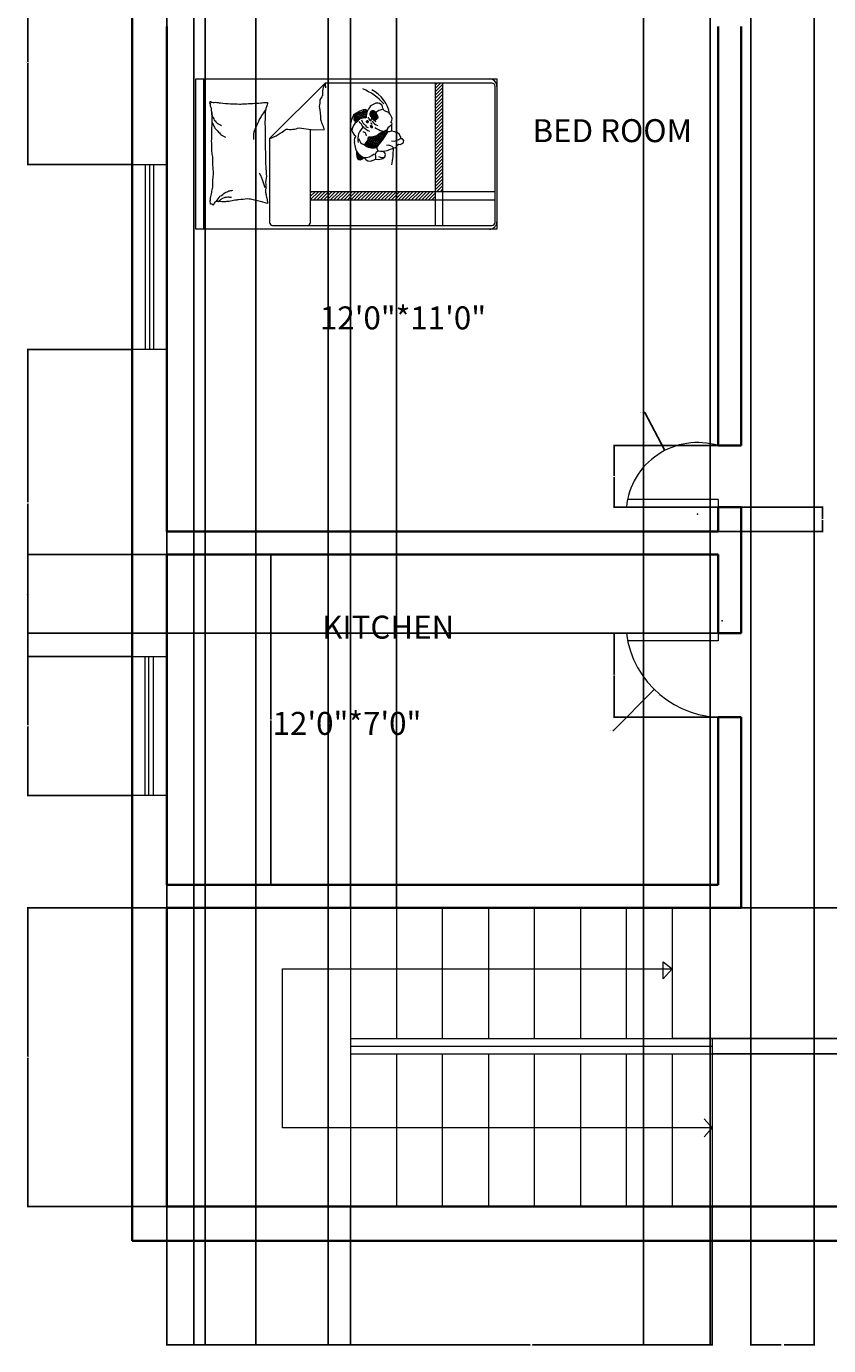
# Model space of a CAD drawing. Units: inches. Extents: x -17 to 1735, y -531 to 60.
# Tile 1 of 27: x -17 to 193, y -531 to -187. Entities that reach past the tile are written whole.
import ezdxf

# ---------------------------------------------------------------- set-up
doc = ezdxf.new("R2010")
doc.units = ezdxf.units.IN
doc.header["$MEASUREMENT"] = 0
for name, color, linetype, lineweight in [('A-ANNO-DIMS', 2, 'Continuous', 18), ('A-AREA-IDEN', 7, 'Continuous', 25), ('A-DOOR', 4, 'Continuous', 18), ('A-FLOR-STRS', 7, 'Continuous', 18), ('A-GLAZ', 4, 'Continuous', 18), ('A-WALL', 7, 'Continuous', 35)]:
    doc.layers.add(name, color=color, linetype=linetype, lineweight=lineweight)
doc.layers.add('A-FURN', color=242, linetype='Continuous', lineweight=18, true_color=0xcd2027)
doc.styles.get("Standard").update_dxf_attribs({"font": 'arial.ttf'})
doc.dimstyles.get("Standard").update_dxf_attribs({"dimtxt": 0.18, "dimasz": 0.18, "dimexe": 0.18, "dimexo": 0.0625, "dimgap": 0.09, "dimtad": 0, "dimtih": 1, "dimtoh": 1, "dimdec": 4, "dimzin": 0, "dimdsep": 46, "dimtxsty": 'Standard', "dimcen": 0.09, "dimadec": 0, "dimazin": 0, "dimtfac": 1, "dimtdec": 4, "dimtofl": 0, "dimtmove": 0, "dimatfit": 3, "dimfxl": 1, "dimtolj": 1, "dimtzin": 0, "dimarcsym": 0})

# ---------------------------------------------------------------- blocks, each defined once
blk = doc.blocks.new('BED-SINGLE-PLAN')
h = blk.add_hatch()
h.set_pattern_fill('ANSI31', color=256, scale=0.196463, angle=90, style=0)
h.set_pattern_definition([(225, (-27.0618, 48.5235), (-0.4410725, 0.4410725), [])])
h.paths.add_polyline_path([(62.55, 9.8), (29.91, 9.8), (29.91, 7.6), (62.55, 7.6)])
h.paths.add_polyline_path([(62.55, 9.8), (64.48, 9.8), (64.48, 38.18), (62.55, 38.18)])
h = blk.add_hatch()
h.set_pattern_fill('ANSI31', color=256, scale=2.357559, angle=112.8083, style=0)
h.set_pattern_definition([(157.808265, (-756.06988, 363.93155), (-0.11130837, -0.27286535), [])])
h.paths.add_polyline_path([(42.9, 28.85), (43.53, 29.05), (44.41, 29.13), (44.47, 29.42), (44.54, 30.16), (44.69, 30.7), (44.07, 30.85), (43.35, 30.52), (41.94, 30.01), (41.58, 29.54), (41.52, 28.62), (41.97, 28.11), (42.32, 28.49)])
h.paths.add_polyline_path([(45.09, 24.15, -0.19505), (43.9, 22.11, 0.242355), (47, 21.35, 0.070869), (50.1, 25.47), (49.89, 25.73), (49.62, 25.88), (48.82, 25.54), (47.87, 25.05), (47.21, 24.51), (46.36, 24.21)])
h = blk.add_hatch()
h.set_pattern_fill('ANSI31', color=256, scale=0.556973, angle=112.8083, style=0)
h.set_pattern_definition([(157.808265, (-714.60694, 367.20017), (-0.0262966024, -0.0644644387), [])])
h.paths.add_polyline_path([(45.8, 27.02), (45.59, 27), (45.47, 26.92), (45.58, 26.73), (45.73, 26.62), (46.03, 26.56), (46.14, 26.64), (46.08, 26.8), (45.97, 26.95)])
h.paths.add_polyline_path([(44.84, 28.32), (44.68, 28.33), (44.51, 28.27), (44.45, 28.18), (44.46, 28.11), (44.56, 28.01), (44.67, 27.9), (44.88, 27.87), (45.01, 27.95), (45.02, 28.12)])
h = blk.add_hatch()
h.set_pattern_fill('ANSI31', color=256, scale=1.392433, angle=112.8083, style=0)
h.set_pattern_definition([(157.808265, (-714.60694, 367.20017), (-0.065741506, -0.161161097), [])])
h.paths.add_polyline_path([(45.75, 29.39), (46.01, 28.9), (46.14, 28.75), (46.34, 28.64), (46.5, 28.59), (46.86, 28.63), (47.26, 28.84), (47.59, 29.2), (47.52, 29.53), (47.21, 29.96), (47.12, 30.29), (46.97, 30.53), (46.54, 30.87), (46.19, 31), (45.76, 30.88), (45.45, 30.56), (45.37, 30.21), (45.4, 29.92), (45.54, 29.52)])
h = blk.add_hatch()
h.set_pattern_fill('ANSI31', color=256, scale=1.178779, angle=112.8083, style=0)
h.set_pattern_definition([(157.808265, (-756.06988, 363.93155), (-0.055654185, -0.136432674), [])])
h.paths.add_polyline_path([(41.9, 20.41), (41.91, 20.39), (41.88, 19.75), (42, 19.04), (42.19, 18.52), (42.51, 18.19), (42.99, 18.18), (43.33, 18.35), (43.64, 18.6), (43.79, 18.72, -0.129501)])
for p, q in [((0, 39.29), (78.59, 39.29)), ((0, 0), (0, 39.29)), ((2.06, 0), (2.06, 39.29)), ((19.2, 23.68), (33.73, 38.18)), ((77.32, 38.18), (33.73, 38.18)), ((62.55, 1.01), (62.55, 38.18)), ((64.48, 1.01), (64.48, 38.18)), ((78.59, 39.29), (78.59, 0)), ((78.11, 1.8), (78.11, 37.39)), ((29.91, 1.8), (29.91, 26.11)), ((19.2, 23.68), (19.2, 1.8)), ((78.59, 0), (0, 0)), ((19.98, 1.01), (77.32, 1.01))]:
    blk.add_line(p, q)
for points in [[(5.25, 7.27, 0.263368), (4.51, 6.17, 0.494818), (3.78, 6.53, 0.049225), (3.71, 7.23, 0.036831), (3.78, 8.16, 0.031893), (4.1, 9.65, -0.035782), (4.37, 10.98, -0.032941), (4.6, 14.51, -0.026564), (4.37, 18.88, -0.017905), (4.16, 20.35, 0.009667), (4.07, 23.11, 0.03204), (4.1, 24.57, -0.018442), (4.22, 27.09, -0.010837), (4.19, 29.64, -0.014624), (4.07, 31.52, -0.111249), (3.78, 32.41, 0.153708), (3.63, 33.07, 0.076444), (3.7, 33.36, 0.215512), (3.78, 33.44, 0.585858), (3.9, 33.33, -0.363489), (4, 33.14, -0.191716), (4.45, 33.14, 0.129675), (5.1, 33.22, 0.01735), (5.76, 33.1, -0.019326), (6.36, 33, -0.018818), (9.04, 32.74, -0.021828), (11.37, 32.7, -0.006204), (12.7, 32.76, -0.001963), (16.9, 33, -0.028341), (18.32, 33.16, 0.117014), (18.67, 33.14, 0.36606), (18.71, 33.09, 0.03973), (18.6, 32.55, 0.048309), (18.38, 32.01, -0.062981), (18.23, 31.59, -0.04058), (18.09, 30.67, -0.014345), (18.01, 28.05, -0.005484), (18.04, 23.12, -0.004707), (18.15, 17.38, -0.008762), (18.26, 15.71, 0.008153), (18.38, 13.91, 0.06251), (18.2, 11.67, -0.078669), (18.12, 9.88, -0.047825), (18.31, 9, 0.034494), (18.6, 7.79, 0.023571), (18.71, 6.79, 0.510228), (18.67, 6.76), (17.49, 7.05), (14.25, 7.86, -0.073041), (13.48, 7.94, -0.023305), (11.08, 7.72, -0.018299), (10.18, 7.56, 0.01097), (8.68, 7.27, 0.042281), (7.34, 7.15, 0.027201), (5.24, 7.27)], [(4, 31.08, -0.088153), (4.14, 29.72, -0.088153), (4.73, 28.5, -0.077547), (5.58, 27.64, -0.077547), (6.65, 27.09)], [(18.15, 31.23, -0.016108), (17.12, 29.7, -0.024599), (16.53, 28.64, -0.009477), (15.62, 26.72, -0.015937), (15.13, 25.54, -0.072521), (14.99, 24.9, -0.033339), (14.98, 23.48)], [(4.22, 27.86, -0.027842), (4.64, 26.92, -0.048685), (4.96, 26.43, -0.023666), (5.91, 25.33, -0.031223), (6.72, 24.58, -0.046801), (7.03, 24.38, -0.023191), (7.68, 24.07)], [(19.2, 23.68, 0.085272), (23.52, 26.17, 0.124044), (26.96, 26.53), (30.71, 25.99), (33.56, 26.06)], [(18.09, 10.82, -0.009729), (17.74, 11.9, -0.009729), (17.34, 12.95, -0.007971), (16.99, 13.81, -0.007971), (16.61, 14.65)], [(5.25, 7.27, 0.077379), (6.25, 8.63, 0.077379), (7.61, 9.63, 0.047525), (8.58, 10.02, 0.047525), (9.6, 10.22)], [(5.88, 7.21, 0.05369), (6.39, 7.77, 0.070312), (6.87, 8.08, 0.015448), (7.21, 8.23, 0.013244), (7.61, 8.38, 0.082127), (8.32, 8.5, 0.064164), (9.23, 8.38)]]:
    blk.add_lwpolyline(points, format="xyb")
for points in [[(43.79, 18.72), (44.04, 18.56), (44.46, 18.12), (44.86, 17.87), (45.53, 17.83), (46.24, 18.04), (46.92, 18.32), (47.57, 18.24), (48.51, 18.4), (48.81, 18.47), (49.3, 18.91), (49.47, 19.49), (49.29, 19.97), (48.92, 20.38), (49.91, 20.56), (51.05, 21.01), (51.55, 21.16), (51.59, 21.33), (51.88, 21.27), (52.46, 21.66), (52.55, 22), (52.94, 22.19), (53.35, 22.15), (53.8, 22.4), (54.07, 22.6), (54.21, 22.84), (54.27, 23.19), (53.95, 23.59), (53.59, 23.67), (53.53, 23.82), (53.51, 24.14), (53.22, 24.49), (53.14, 24.75), (52.57, 25.26), (52.25, 25.24), (51.94, 25.49), (50.98, 25.59), (50.47, 25.47), (50.13, 25.44), (49.89, 25.73), (49.62, 25.88), (49.97, 26.17), (50.19, 26.42), (50.21, 26.66), (50.65, 26.93), (50.88, 27.18), (51.12, 27.37), (51.24, 27.65), (51.14, 27.82), (50.96, 27.83), (50.98, 28.05), (51.12, 28.43), (51.19, 28.96), (51.17, 29.16), (50.93, 29.59), (50.71, 30.03), (50.42, 30.38), (49.9, 30.7), (49.25, 30.9), (49.09, 31.16), (48.83, 31.61), (48.74, 31.98), (48.58, 32.42), (47.95, 32.87), (47.57, 32.94), (46.99, 32.91), (46.24, 32.59), (45.6, 32.26), (45.31, 31.84), (44.99, 31.21), (44.78, 31), (44.17, 31.25), (43.66, 31.18), (42.75, 30.83), (42.33, 30.56), (41.65, 30.22), (41.1, 29.84), (40.84, 29.19), (40.62, 28.57), (40.38, 27.67), (40.38, 26.55), (40.44, 26.19), (40.7, 25.86), (40.89, 25.34), (41.33, 24.64), (41.74, 24.31), (41.36, 23.8), (41.32, 23.27), (41.4, 23.13), (41.29, 22.64), (41.54, 21.48), (41.64, 21.02), (41.71, 20.72), (41.85, 20.54), (41.91, 20.39), (41.88, 19.75), (42, 19.04), (42.19, 18.52), (42.51, 18.19), (42.99, 18.18), (43.33, 18.35), (43.64, 18.6), (43.79, 18.72)], [(41.81, 27.96), (41.3, 28.55), (41.37, 29.62), (41.81, 30.2), (43.27, 30.72), (44.05, 31.08), (44.74, 30.91)], [(41.97, 28.11), (41.52, 28.62), (41.58, 29.54), (41.94, 30.01), (43.35, 30.52), (44.07, 30.85), (44.69, 30.7)], [(44.78, 31), (44.54, 30.16), (44.47, 29.42), (44.41, 29.13), (43.53, 29.05), (42.9, 28.85), (42.32, 28.49), (41.97, 28.11)], [(44.67, 27.9), (44.88, 27.87), (45.01, 27.95), (45.02, 28.12), (44.84, 28.32), (44.68, 28.33), (44.51, 28.27), (44.45, 28.18), (44.46, 28.11), (44.56, 28.01), (44.67, 27.9)], [(45.75, 29.39), (46.01, 28.9), (46.14, 28.75), (46.34, 28.64), (46.5, 28.59), (46.86, 28.63), (47.26, 28.84), (47.59, 29.2), (47.52, 29.53), (47.21, 29.96), (47.12, 30.29), (46.97, 30.53), (46.54, 30.87), (46.19, 31), (45.76, 30.88), (45.45, 30.56), (45.37, 30.21), (45.4, 29.92), (45.54, 29.52), (45.75, 29.39)], [(45.09, 24.15), (46.36, 24.21), (47.21, 24.51), (47.87, 25.05), (48.82, 25.54), (49.62, 25.88)], [(45.73, 26.62), (46.03, 26.56), (46.14, 26.64), (46.08, 26.8), (45.97, 26.95), (45.8, 27.02), (45.59, 27), (45.47, 26.92), (45.58, 26.73), (45.73, 26.62)], [(46.92, 18.32), (46.96, 18.99), (46.83, 19.65), (47.14, 20.19), (47.67, 20.47), (48.14, 20.41), (48.92, 20.38)], [(78.11, 9.8), (29.91, 9.8)], [(78.11, 7.6), (29.91, 7.6)]]:
    blk.add_lwpolyline(points)
for centre, radius, start, end in [((38, 35.55), 5.01, 148.4201, 187.4443), ((39.59, 38.03), 5.86, 178.5957, 190.5745), ((76.62, 37.33), 1.96, 0, 90), ((77.32, 37.39), 0.786, 0, 90), ((30.16, 35.71), 2.97, 320.6139, 344.2839), ((38.03, 23.16), 14.6, 41.0314, 67.8934), ((42.02, 28.67), 8.66, 9.4371, 63.5432), ((26.72, 33.64), 5.74, 344.2839, 1.7887), ((10.08, 27.94), 22.56, 1.7887, 10.5945), ((49.55, 27.35), 4.08, 98.3054, 168.9473), ((26.25, 26.33), 6.78, 10.5945, 19.9478), ((19.4, 20.92), 15.06, 19.9478, 26.2172), ((44.35, 25.28), 3.69, 130.0646, 171.0184), ((40.73, 25.75), 3, 17.6284, 51.9822), ((45.01, 28.9), 1.81, 191.014, 241.9838), ((46.38, 29.75), 1.54, 196.6236, 237.032), ((46.1, 27.86), 0.431, 180.1097, 257.3601), ((46.45, 29.64), 0.695, 97.7782, 185.1837), ((45.99, 30.23), 0.379, 14.3938, 104.927), ((48.22, 29.75), 2.7, 214.8006, 254.2713), ((46.73, 29.37), 0.572, 4.9536, 167.0589), ((54.94, 39.79), 14.12, 231.9927, 235.4886), ((46.6, 29.87), 0.512, 10.7395, 118.1073), ((46.27, 23.6), 4.03, 126.6141, 193.9334), ((43.31, 24.26), 1.25, 5.5542, 75.9589), ((47.07, 29.65), 4.44, 223.4778, 246.0857), ((41.98, 24.59), 3.13, 307.7547, 351.9024), ((44.99, 27.32), 0.729, 184.2478, 266.558), ((49.36, 29.79), 4.14, 230.1138, 260.2426), ((34.07, 34.29), 18.29, 314.9707, 331.1855), ((11.77, 25.26), 39.39, 0.4734, 3.0628), ((46.04, 23.16), 4.97, 209.3586, 243.0552), ((44.61, 24.23), 2.23, 194.7325, 251.4551), ((46.2, 24.74), 3.49, 228.8697, 283.3627), ((48.1, 21.24), 0.883, 163.0797, 240.2757), ((50.18, 20.2), 1.73, 36.8303, 104.4951), ((51.66, 25.7), 2.65, 256.5554, 314.9062), ((29.44, 21.14), 22.11, 348.8153, 0.0463), ((44.02, 22.54), 3.83, 266.6283, 311.5254), ((48.58, 20.29), 1.56, 234.8325, 297.5513), ((19.98, 1.8), 0.786, 180, 270), ((29.12, 1.8), 0.786, 270, 0), ((76.62, 1.96), 1.96, 270, 0), ((77.32, 1.8), 0.786, 270, 0)]:
    blk.add_arc(centre, radius, start, end)
blk = doc.blocks.new('WIN-FRAME-48IN')
for p, q in [((3.31, 48.33), (3.31, 0)), ((5.59, 0), (5.59, 48.33))]:
    blk.add_line(p, q)
blk.add_lwpolyline([(0, 48.33), (9, 48.33), (9, 0), (0, 0)], close=True)
blk = doc.blocks.new('*D11')
at = {"layer": 'A-ANNO-DIMS', "color": 0, "lineweight": -2, "transparency": 16777216}
for p, q in [((20.06, 23.17), (20.06, -531.46)), ((62.23, 23.17), (62.23, -531.46)), ((20.24, -531.28), (40.75, -531.28)), ((62.05, -531.28), (41.54, -531.28))]:
    blk.add_line(p, q, dxfattribs=at)
at = {"layer": 'A-ANNO-DIMS', "color": 0, "transparency": 16777216}
for points in [[(20.24, -531.25), (20.24, -531.31), (20.06, -531.28)], [(62.05, -531.25), (62.05, -531.31), (62.23, -531.28)]]:
    blk.add_solid(points, dxfattribs=at)
at = {"layer": 'Defpoints', "color": 0, "transparency": 16777216}
for p in [(20.06, 23.23), (62.23, 23.23), (62.23, -531.28)]:
    blk.add_point(p, dxfattribs=at)
at = {"layer": 'A-ANNO-DIMS', "color": 0, "transparency": 16777216, "insert": (41.15, -531.28), "char_height": 0.18, "attachment_point": 5}
blk.add_mtext('\\A1;42.17', dxfattribs=at)
blk = doc.blocks.new('*D15')
at = {"layer": 'A-ANNO-DIMS', "color": 0, "lineweight": -2, "transparency": 16777216}
for p, q in [((11, -169.55), (-16.4, -169.55)), ((-16.22, -169.73), (-16.22, -196.03)), ((-16.22, -222.7), (-16.22, -196.39)), ((11, -222.88), (-16.4, -222.88))]:
    blk.add_line(p, q, dxfattribs=at)
at = {"layer": 'A-ANNO-DIMS', "color": 0, "transparency": 16777216}
for points in [[(-16.25, -169.73), (-16.19, -169.73), (-16.22, -169.55)], [(-16.25, -222.7), (-16.19, -222.7), (-16.22, -222.88)]]:
    blk.add_solid(points, dxfattribs=at)
at = {"layer": 'Defpoints', "color": 0, "transparency": 16777216}
for p in [(11.06, -169.55), (-16.22, -222.88), (11.06, -222.88)]:
    blk.add_point(p, dxfattribs=at)
at = {"layer": 'A-ANNO-DIMS', "color": 0, "transparency": 16777216, "insert": (-16.22, -196.21), "char_height": 0.18, "attachment_point": 5}
blk.add_mtext('\\A1;53.33', dxfattribs=at)
blk = doc.blocks.new('*D16')
at = {"layer": 'A-ANNO-DIMS', "color": 0, "lineweight": -2, "transparency": 16777216}
for p, q in [((11, -271.2), (-16.4, -271.2)), ((-16.22, -271.38), (-16.22, -311.12)), ((-16.22, -351.23), (-16.22, -311.49)), ((10.91, -351.41), (-16.4, -351.41))]:
    blk.add_line(p, q, dxfattribs=at)
at = {"layer": 'A-ANNO-DIMS', "color": 0, "transparency": 16777216}
for points in [[(-16.25, -271.38), (-16.19, -271.38), (-16.22, -271.2)], [(-16.25, -351.23), (-16.19, -351.23), (-16.22, -351.41)]]:
    blk.add_solid(points, dxfattribs=at)
at = {"layer": 'Defpoints', "color": 0, "transparency": 16777216}
for p in [(11.06, -271.2), (-16.22, -351.41), (10.98, -351.41)]:
    blk.add_point(p, dxfattribs=at)
at = {"layer": 'A-ANNO-DIMS', "color": 0, "transparency": 16777216, "insert": (-16.22, -311.3), "char_height": 0.18, "attachment_point": 5}
blk.add_mtext('\\A1;80.2', dxfattribs=at)
blk = doc.blocks.new('*D17')
at = {"layer": 'A-ANNO-DIMS', "color": 0, "lineweight": -2, "transparency": 16777216}
for p, q in [((10.91, -351.41), (-16.4, -351.41)), ((-16.22, -351.59), (-16.22, -369.37)), ((-16.22, -387.51), (-16.22, -369.73)), ((10.91, -387.69), (-16.4, -387.69))]:
    blk.add_line(p, q, dxfattribs=at)
at = {"layer": 'A-ANNO-DIMS', "color": 0, "transparency": 16777216}
for points in [[(-16.25, -351.59), (-16.19, -351.59), (-16.22, -351.41)], [(-16.25, -387.51), (-16.19, -387.51), (-16.22, -387.69)]]:
    blk.add_solid(points, dxfattribs=at)
at = {"layer": 'Defpoints', "color": 0, "transparency": 16777216}
for p in [(10.98, -351.41), (-16.22, -387.69), (10.98, -387.69)]:
    blk.add_point(p, dxfattribs=at)
at = {"layer": 'A-ANNO-DIMS', "color": 0, "transparency": 16777216, "insert": (-16.22, -369.55), "char_height": 0.18, "attachment_point": 5}
blk.add_mtext('\\A1;36.28', dxfattribs=at)
blk = doc.blocks.new('*D30')
at = {"layer": 'A-ANNO-DIMS', "color": 0, "lineweight": -2, "transparency": 16777216}
for p, q in [((144.53, -126.83), (144.53, -531.46)), ((161.94, -126.83), (161.94, -531.46)), ((144.71, -531.28), (152.87, -531.28)), ((161.76, -531.28), (153.6, -531.28))]:
    blk.add_line(p, q, dxfattribs=at)
at = {"layer": 'A-ANNO-DIMS', "color": 0, "transparency": 16777216}
for points in [[(144.71, -531.25), (144.71, -531.31), (144.53, -531.28)], [(161.76, -531.25), (161.76, -531.31), (161.94, -531.28)]]:
    blk.add_solid(points, dxfattribs=at)
at = {"layer": 'Defpoints', "color": 0, "transparency": 16777216}
for p in [(144.53, -126.77), (161.94, -126.77), (161.94, -531.28)]:
    blk.add_point(p, dxfattribs=at)
at = {"layer": 'A-ANNO-DIMS', "color": 0, "transparency": 16777216, "insert": (153.23, -531.28), "char_height": 0.18, "attachment_point": 5}
blk.add_mtext('\\A1;17.41', dxfattribs=at)
blk = doc.blocks.new('*D31')
at = {"layer": 'A-ANNO-DIMS', "color": 0, "lineweight": -2, "transparency": 16777216}
for p, q in [((172.55, -126.83), (172.55, -531.46)), ((189.13, -126.83), (189.13, -531.46)), ((172.73, -531.28), (180.46, -531.28)), ((188.95, -531.28), (181.23, -531.28))]:
    blk.add_line(p, q, dxfattribs=at)
at = {"layer": 'A-ANNO-DIMS', "color": 0, "transparency": 16777216}
for points in [[(172.73, -531.25), (172.73, -531.31), (172.55, -531.28)], [(188.95, -531.25), (188.95, -531.31), (189.13, -531.28)]]:
    blk.add_solid(points, dxfattribs=at)
at = {"layer": 'Defpoints', "color": 0, "transparency": 16777216}
for p in [(172.55, -126.77), (189.13, -126.77), (189.13, -531.28)]:
    blk.add_point(p, dxfattribs=at)
at = {"layer": 'A-ANNO-DIMS', "color": 0, "transparency": 16777216, "insert": (180.84, -531.28), "char_height": 0.18, "attachment_point": 5}
blk.add_mtext('\\A1;16.58', dxfattribs=at)
blk = doc.blocks.new('*D33')
at = {"layer": 'A-ANNO-DIMS', "color": 0, "lineweight": -2, "transparency": 16777216}
for p, q in [((164, -296.3), (136.68, -296.3)), ((136.86, -296.48), (136.86, -304.18)), ((136.86, -312.24), (136.86, -304.54)), ((164, -312.42), (136.68, -312.42))]:
    blk.add_line(p, q, dxfattribs=at)
at = {"layer": 'A-ANNO-DIMS', "color": 0, "transparency": 16777216}
for points in [[(136.83, -296.48), (136.89, -296.48), (136.86, -296.3)], [(136.83, -312.24), (136.89, -312.24), (136.86, -312.42)]]:
    blk.add_solid(points, dxfattribs=at)
at = {"layer": 'Defpoints', "color": 0, "transparency": 16777216}
for p in [(136.86, -296.3), (164.06, -296.3), (164.06, -312.42)]:
    blk.add_point(p, dxfattribs=at)
at = {"layer": 'A-ANNO-DIMS', "color": 0, "transparency": 16777216, "insert": (136.86, -304.36), "char_height": 0.18, "attachment_point": 5}
blk.add_mtext('\\A1;16.116', dxfattribs=at)
blk = doc.blocks.new('*D34')
at = {"layer": 'A-ANNO-DIMS', "color": 0, "lineweight": -2, "transparency": 16777216}
for p, q in [((164.12, -312.42), (191.44, -312.42)), ((191.26, -312.6), (191.26, -315.41)), ((191.26, -318.59), (191.26, -315.78)), ((164.12, -318.77), (191.44, -318.77))]:
    blk.add_line(p, q, dxfattribs=at)
at = {"layer": 'A-ANNO-DIMS', "color": 0, "transparency": 16777216}
for points in [[(191.23, -312.6), (191.29, -312.6), (191.26, -312.42)], [(191.23, -318.59), (191.29, -318.59), (191.26, -318.77)]]:
    blk.add_solid(points, dxfattribs=at)
at = {"layer": 'Defpoints', "color": 0, "transparency": 16777216}
for p in [(164.06, -312.42), (164.06, -318.77), (191.26, -318.77)]:
    blk.add_point(p, dxfattribs=at)
at = {"layer": 'A-ANNO-DIMS', "color": 0, "transparency": 16777216, "insert": (191.26, -315.59), "char_height": 0.18, "attachment_point": 5}
blk.add_mtext('\\A1;6.351', dxfattribs=at)
blk = doc.blocks.new('*D35')
at = {"layer": 'A-ANNO-DIMS', "color": 0, "lineweight": -2, "transparency": 16777216}
for p, q in [((164, -324.77), (-16.4, -324.77)), ((-16.22, -324.95), (-16.22, -334.86)), ((-16.22, -345.14), (-16.22, -335.23)), ((164, -345.32), (-16.4, -345.32))]:
    blk.add_line(p, q, dxfattribs=at)
at = {"layer": 'A-ANNO-DIMS', "color": 0, "transparency": 16777216}
for points in [[(-16.25, -324.95), (-16.19, -324.95), (-16.22, -324.77)], [(-16.25, -345.14), (-16.19, -345.14), (-16.22, -345.32)]]:
    blk.add_solid(points, dxfattribs=at)
at = {"layer": 'Defpoints', "color": 0, "transparency": 16777216}
for p in [(-16.22, -324.77), (164.06, -324.77), (164.06, -345.32)]:
    blk.add_point(p, dxfattribs=at)
at = {"layer": 'A-ANNO-DIMS', "color": 0, "transparency": 16777216, "insert": (-16.22, -335.04), "char_height": 0.18, "attachment_point": 5}
blk.add_mtext('\\A1;20.553', dxfattribs=at)
blk = doc.blocks.new('*D36')
at = {"layer": 'A-ANNO-DIMS', "color": 0, "lineweight": -2, "transparency": 16777216}
for p, q in [((164, -345.32), (136.68, -345.32)), ((136.86, -345.5), (136.86, -356.1)), ((136.86, -367.06), (136.86, -356.46)), ((164, -367.24), (136.68, -367.24))]:
    blk.add_line(p, q, dxfattribs=at)
at = {"layer": 'A-ANNO-DIMS', "color": 0, "transparency": 16777216}
for points in [[(136.83, -345.5), (136.89, -345.5), (136.86, -345.32)], [(136.83, -367.06), (136.89, -367.06), (136.86, -367.24)]]:
    blk.add_solid(points, dxfattribs=at)
at = {"layer": 'Defpoints', "color": 0, "transparency": 16777216}
for p in [(136.86, -345.32), (164.06, -345.32), (164.06, -367.24)]:
    blk.add_point(p, dxfattribs=at)
at = {"layer": 'A-ANNO-DIMS', "color": 0, "transparency": 16777216, "insert": (136.86, -356.28), "char_height": 0.18, "attachment_point": 5}
blk.add_mtext('\\A1;21.923', dxfattribs=at)
blk = doc.blocks.new('*D42')
at = {"layer": 'A-ANNO-DIMS', "color": 0, "lineweight": -2, "transparency": 16777216}
for p, q in [((20.12, -324.77), (47.44, -324.77)), ((47.26, -324.95), (47.26, -367.74)), ((47.26, -410.9), (47.26, -368.11)), ((20.12, -411.08), (47.44, -411.08))]:
    blk.add_line(p, q, dxfattribs=at)
at = {"layer": 'A-ANNO-DIMS', "color": 0, "transparency": 16777216}
for points in [[(47.23, -324.95), (47.29, -324.95), (47.26, -324.77)], [(47.23, -410.9), (47.29, -410.9), (47.26, -411.08)]]:
    blk.add_solid(points, dxfattribs=at)
at = {"layer": 'Defpoints', "color": 0, "transparency": 16777216}
for p in [(20.06, -324.77), (20.06, -411.08), (47.26, -411.08)]:
    blk.add_point(p, dxfattribs=at)
at = {"layer": 'A-ANNO-DIMS', "color": 0, "transparency": 16777216, "insert": (47.26, -367.92), "char_height": 0.18, "attachment_point": 5}
blk.add_mtext('\\A1;86.31', dxfattribs=at)
blk = doc.blocks.new('*D45')
at = {"layer": 'A-ANNO-DIMS', "color": 0, "lineweight": -2, "transparency": 16777216}
for p, q in [((27.16, -164.32), (27.16, -531.46)), ((43.3, -164.32), (43.3, -531.46)), ((27.34, -531.28), (34.85, -531.28)), ((43.12, -531.28), (35.62, -531.28))]:
    blk.add_line(p, q, dxfattribs=at)
at = {"layer": 'A-ANNO-DIMS', "color": 0, "transparency": 16777216}
for points in [[(27.34, -531.25), (27.34, -531.31), (27.16, -531.28)], [(43.12, -531.25), (43.12, -531.31), (43.3, -531.28)]]:
    blk.add_solid(points, dxfattribs=at)
at = {"layer": 'Defpoints', "color": 0, "transparency": 16777216}
for p in [(27.16, -164.25), (43.3, -164.25), (43.3, -531.28)]:
    blk.add_point(p, dxfattribs=at)
at = {"layer": 'A-ANNO-DIMS', "color": 0, "transparency": 16777216, "insert": (35.23, -531.28), "char_height": 0.18, "attachment_point": 5}
blk.add_mtext('\\A1;16.14', dxfattribs=at)
blk = doc.blocks.new('*D46')
at = {"layer": 'A-ANNO-DIMS', "color": 0, "lineweight": -2, "transparency": 16777216}
for p, q in [((30.1, -177.39), (30.1, -531.46)), ((20.06, -180.83), (20.06, -531.46)), ((20.24, -531.28), (24.62, -531.28)), ((29.92, -531.28), (25.53, -531.28))]:
    blk.add_line(p, q, dxfattribs=at)
at = {"layer": 'A-ANNO-DIMS', "color": 0, "transparency": 16777216}
for points in [[(20.24, -531.25), (20.24, -531.31), (20.06, -531.28)], [(29.92, -531.25), (29.92, -531.31), (30.1, -531.28)]]:
    blk.add_solid(points, dxfattribs=at)
at = {"layer": 'Defpoints', "color": 0, "transparency": 16777216}
for p in [(30.1, -177.33), (20.06, -180.77), (30.1, -531.28)]:
    blk.add_point(p, dxfattribs=at)
at = {"layer": 'A-ANNO-DIMS', "color": 0, "transparency": 16777216, "insert": (25.08, -531.28), "char_height": 0.18, "attachment_point": 5}
blk.add_mtext('\\A1;10.034', dxfattribs=at)
blk = doc.blocks.new('*D47')
at = {"layer": 'A-ANNO-DIMS', "color": 0, "lineweight": -2, "transparency": 16777216}
for p, q in [((20, -417.08), (-16.4, -417.08)), ((-16.22, -417.26), (-16.22, -455.9)), ((-16.22, -494.9), (-16.22, -456.26)), ((20, -495.08), (-16.4, -495.08))]:
    blk.add_line(p, q, dxfattribs=at)
at = {"layer": 'A-ANNO-DIMS', "color": 0, "transparency": 16777216}
for points in [[(-16.25, -417.26), (-16.19, -417.26), (-16.22, -417.08)], [(-16.25, -494.9), (-16.19, -494.9), (-16.22, -495.08)]]:
    blk.add_solid(points, dxfattribs=at)
at = {"layer": 'Defpoints', "color": 0, "transparency": 16777216}
for p in [(-16.22, -417.08), (20.06, -417.08), (20.06, -495.08)]:
    blk.add_point(p, dxfattribs=at)
at = {"layer": 'A-ANNO-DIMS', "color": 0, "transparency": 16777216, "insert": (-16.22, -456.08), "char_height": 0.18, "attachment_point": 5}
blk.add_mtext('\\A1;78', dxfattribs=at)
blk = doc.blocks.new('*D48')
at = {"layer": 'A-ANNO-DIMS', "color": 0, "lineweight": -2, "transparency": 16777216}
for p, q in [((20.06, -495.14), (20.06, -531.46)), ((68.06, -495.14), (68.06, -531.46)), ((20.24, -531.28), (43.84, -531.28)), ((67.88, -531.28), (44.28, -531.28))]:
    blk.add_line(p, q, dxfattribs=at)
at = {"layer": 'A-ANNO-DIMS', "color": 0, "transparency": 16777216}
for points in [[(20.24, -531.25), (20.24, -531.31), (20.06, -531.28)], [(67.88, -531.25), (67.88, -531.31), (68.06, -531.28)]]:
    blk.add_solid(points, dxfattribs=at)
at = {"layer": 'Defpoints', "color": 0, "transparency": 16777216}
for p in [(20.06, -495.08), (68.06, -495.08), (68.06, -531.28)]:
    blk.add_point(p, dxfattribs=at)
at = {"layer": 'A-ANNO-DIMS', "color": 0, "transparency": 16777216, "insert": (44.06, -531.28), "char_height": 0.18, "attachment_point": 5}
blk.add_mtext('\\A1;48', dxfattribs=at)
blk = doc.blocks.new('*D49')
at = {"layer": 'A-ANNO-DIMS', "color": 0, "lineweight": -2, "transparency": 16777216}
for p, q in [((68.06, -495.14), (68.06, -531.46)), ((162.47, -495.14), (162.47, -531.46)), ((68.24, -531.28), (114.94, -531.28)), ((162.29, -531.28), (115.59, -531.28))]:
    blk.add_line(p, q, dxfattribs=at)
at = {"layer": 'A-ANNO-DIMS', "color": 0, "transparency": 16777216}
for points in [[(68.24, -531.25), (68.24, -531.31), (68.06, -531.28)], [(162.29, -531.25), (162.29, -531.31), (162.47, -531.28)]]:
    blk.add_solid(points, dxfattribs=at)
at = {"layer": 'Defpoints', "color": 0, "transparency": 16777216}
for p in [(68.06, -495.08), (162.47, -495.08), (162.47, -531.28)]:
    blk.add_point(p, dxfattribs=at)
at = {"layer": 'A-ANNO-DIMS', "color": 0, "transparency": 16777216, "insert": (115.26, -531.28), "char_height": 0.18, "attachment_point": 5}
blk.add_mtext('\\A1;94.4', dxfattribs=at)
blk = doc.blocks.new('*D50')
at = {"layer": 'A-ANNO-DIMS', "color": 0, "lineweight": -2, "transparency": 16777216}
for p, q in [((68.06, -417.02), (68.06, 59.62)), ((68.24, 59.44), (73.85, 59.44)), ((79.88, 59.44), (74.27, 59.44)), ((80.06, -417.02), (80.06, 59.62))]:
    blk.add_line(p, q, dxfattribs=at)
at = {"layer": 'A-ANNO-DIMS', "color": 0, "transparency": 16777216}
for points in [[(68.24, 59.47), (68.24, 59.41), (68.06, 59.44)], [(79.88, 59.47), (79.88, 59.41), (80.06, 59.44)]]:
    blk.add_solid(points, dxfattribs=at)
at = {"layer": 'Defpoints', "color": 0, "transparency": 16777216}
for p in [(80.06, 59.44), (68.06, -417.08), (80.06, -417.08)]:
    blk.add_point(p, dxfattribs=at)
at = {"layer": 'A-ANNO-DIMS', "color": 0, "transparency": 16777216, "insert": (74.06, 59.44), "char_height": 0.18, "attachment_point": 5}
blk.add_mtext('\\A1;12', dxfattribs=at)
blk = doc.blocks.new('*D51')
at = {"layer": 'A-ANNO-DIMS', "color": 0, "lineweight": -2, "transparency": 16777216}
for p, q in [((152.12, -417.08), (356.44, -417.08)), ((356.26, -417.26), (356.26, -433.97)), ((356.26, -451.04), (356.26, -434.33)), ((152.12, -451.22), (356.44, -451.22))]:
    blk.add_line(p, q, dxfattribs=at)
at = {"layer": 'A-ANNO-DIMS', "color": 0, "transparency": 16777216}
for points in [[(356.23, -417.26), (356.29, -417.26), (356.26, -417.08)], [(356.23, -451.04), (356.29, -451.04), (356.26, -451.22)]]:
    blk.add_solid(points, dxfattribs=at)
at = {"layer": 'Defpoints', "color": 0, "transparency": 16777216}
for p in [(152.06, -417.08), (152.06, -451.22), (356.26, -451.22)]:
    blk.add_point(p, dxfattribs=at)
at = {"layer": 'A-ANNO-DIMS', "color": 0, "transparency": 16777216, "insert": (356.26, -434.15), "char_height": 0.18, "attachment_point": 5}
blk.add_mtext('\\A1;34.14', dxfattribs=at)
blk = doc.blocks.new('*D52')
at = {"layer": 'A-ANNO-DIMS', "color": 0, "lineweight": -2, "transparency": 16777216}
for p, q in [((162.53, -455.22), (356.44, -455.22)), ((356.26, -455.4), (356.26, -474.97)), ((356.26, -494.9), (356.26, -475.33)), ((162.53, -495.08), (356.44, -495.08))]:
    blk.add_line(p, q, dxfattribs=at)
at = {"layer": 'A-ANNO-DIMS', "color": 0, "transparency": 16777216}
for points in [[(356.23, -455.4), (356.29, -455.4), (356.26, -455.22)], [(356.23, -494.9), (356.29, -494.9), (356.26, -495.08)]]:
    blk.add_solid(points, dxfattribs=at)
at = {"layer": 'Defpoints', "color": 0, "transparency": 16777216}
for p in [(162.47, -455.22), (162.47, -495.08), (356.26, -495.08)]:
    blk.add_point(p, dxfattribs=at)
at = {"layer": 'A-ANNO-DIMS', "color": 0, "transparency": 16777216, "insert": (356.26, -475.15), "char_height": 0.18, "attachment_point": 5}
blk.add_mtext('\\A1;39.86', dxfattribs=at)
blk = doc.blocks.new('*D56')
at = {"layer": 'A-ANNO-DIMS', "color": 0, "lineweight": -2, "transparency": 16777216}
for p, q in [((144.74, -287.64), (144.92, -287.64)), ((144.92, -287.64), (149.99, -297.44)), ((158.58, -314.2), (158.76, -314.2)), ((158.67, -314.29), (158.67, -314.11))]:
    blk.add_line(p, q, dxfattribs=at)
at = {"layer": 'A-ANNO-DIMS', "color": 0, "transparency": 16777216}
blk.add_solid([(150.02, -297.43), (149.96, -297.45), (150.07, -297.6)], dxfattribs=at)
at = {"layer": 'Defpoints', "color": 0, "transparency": 16777216}
for p in [(150.07, -297.6), (158.67, -314.2)]:
    blk.add_point(p, dxfattribs=at)
at = {"layer": 'A-ANNO-DIMS', "color": 0, "transparency": 16777216, "insert": (144.19, -287.64), "char_height": 0.18, "attachment_point": 5}
blk.add_mtext('\\A1;R18.693', dxfattribs=at)
blk = doc.blocks.new('*D57')
at = {"layer": 'A-ANNO-DIMS', "color": 0, "lineweight": -2, "transparency": 16777216}
for p, q in [((164.95, -342.07), (165.13, -342.07)), ((165.04, -342.16), (165.04, -341.98)), ((136.73, -370.76), (147.22, -360.13)), ((136.55, -370.76), (136.73, -370.76))]:
    blk.add_line(p, q, dxfattribs=at)
at = {"layer": 'A-ANNO-DIMS', "color": 0, "transparency": 16777216}
blk.add_solid([(147.2, -360.11), (147.24, -360.15), (147.35, -360)], dxfattribs=at)
at = {"layer": 'Defpoints', "color": 0, "transparency": 16777216}
for p in [(165.04, -342.07), (147.35, -360)]:
    blk.add_point(p, dxfattribs=at)
at = {"layer": 'A-ANNO-DIMS', "color": 0, "transparency": 16777216, "insert": (136.07, -370.76), "char_height": 0.18, "attachment_point": 5}
blk.add_mtext('\\A1;R25.19', dxfattribs=at)

msp = doc.modelspace()

# ---------------------------------------------------------------- linework, layer by layer
at = {"layer": 'A-DOOR'}
for p, q in [((164.0618, -312.4176), (140.0618, -312.4176)), ((164.0618, -310.4176), (140.3633, -310.4176)), ((164.0618, -310.4176), (164.0618, -312.4176)), ((164.0618, -345.3213), (140.0618, -345.3213)), ((164.0618, -347.3213), (140.4044, -347.3213)), ((164.0618, -345.3213), (164.0618, -347.3213))]:
    msp.add_line(p, q, dxfattribs=at)
for centre, radius, start, end in [((158.6693, -314.1999), 18.6927, 73.232883, 174.528677), ((165.0435, -342.0715), 25.1923, 187.411932, 272.233429)]:
    msp.add_arc(centre, radius, start, end, dxfattribs=at)
at = {"layer": 'A-FLOR-STRS'}
for p, q in [((68.0618, -417.0795), (68.0618, -495.0795)), ((80.0618, -417.0795), (80.0618, -451.2168)), ((92.0618, -417.0795), (104.0618, -417.0795)), ((92.0618, -451.2168), (92.0618, -417.0795)), ((104.0618, -417.0795), (104.0618, -451.2168)), ((116.0618, -417.0795), (128.0618, -417.0795)), ((116.0618, -451.2168), (116.0618, -417.0795)), ((128.0618, -417.0795), (128.0618, -451.2168)), ((140.0618, -417.0795), (152.0618, -417.0795)), ((140.0618, -451.2168), (140.0618, -417.0795)), ((152.0618, -417.0795), (152.0618, -451.2168)), ((50.3039, -474.5978), (50.3039, -433.0377)), ((50.3039, -433.0377), (152.0618, -433.0377)), ((149.673, -435.5913), (149.673, -431.2211)), ((149.673, -431.2211), (152.0618, -433.0377)), ((152.0618, -433.0377), (149.673, -435.5913)), ((68.0618, -451.2168), (162.4671, -451.2168)), ((162.4671, -451.2168), (162.4671, -495.0795)), ((68.0618, -453.2168), (162.4671, -453.2168)), ((68.0618, -455.2168), (162.4671, -455.2168)), ((80.0618, -455.2168), (80.0618, -495.0795)), ((92.0618, -495.0795), (92.0618, -455.2168)), ((104.0618, -455.2168), (104.0618, -495.0795)), ((116.0618, -495.0795), (116.0618, -455.2168)), ((128.0618, -455.2168), (128.0618, -495.0795)), ((140.0618, -495.0795), (140.0618, -455.2168)), ((152.0618, -455.2168), (152.0618, -495.0795)), ((162.4671, -474.5978), (50.3039, -474.5978)), ((162.4671, -474.5978), (160.4201, -472.2475)), ((160.4201, -476.933), (162.4671, -474.5978)), ((80.0618, -495.0795), (92.0618, -495.0795)), ((104.0618, -495.0795), (116.0618, -495.0795)), ((128.0618, -495.0795), (140.0618, -495.0795))]:
    msp.add_line(p, q, dxfattribs=at)
at = {"layer": 'A-GLAZ'}
for p, q in [((15.5227, -222.8758), (15.5227, -271.2016)), ((14.2873, -351.4056), (14.2873, -387.689)), ((15.2956, -351.4056), (15.2956, -387.689)), ((16.569, -387.689), (16.569, -351.4056)), ((19.9763, -387.689), (10.9763, -387.689))]:
    msp.add_line(p, q, dxfattribs=at)
msp.add_lwpolyline([(10.9763, -387.689), (10.9763, -351.4056), (19.9763, -351.4056), (19.9763, -387.689)], dxfattribs=at)
at = {"layer": 'A-WALL'}
for p, q in [((11.0618, -141.0795), (11.0618, -195.0795)), ((20.0618, -195.0795), (20.0618, -186.7685)), ((164.0618, -186.7685), (164.0618, -296.302)), ((170.0618, -186.7685), (170.0618, -296.302)), ((11.0618, -195.0795), (11.0618, -327.0795)), ((20.0618, -195.0795), (20.0618, -318.7685)), ((20.0618, -262.8906), (20.0618, -271.2016)), ((170.0618, -296.302), (164.0618, -296.302)), ((164.0618, -312.4176), (170.0618, -312.4176)), ((164.0618, -312.4176), (164.0618, -318.7685)), ((170.0618, -312.4176), (170.0618, -329.0197)), ((164.0618, -318.7685), (20.0618, -318.7685)), ((11.0618, -327.0795), (11.0618, -411.0795)), ((164.0618, -324.7685), (20.0618, -324.7685)), ((20.0618, -324.7685), (20.0618, -327.0795)), ((20.0618, -327.0795), (20.0618, -411.0795)), ((164.0618, -329.0197), (164.0618, -324.7685)), ((170.0618, -329.0197), (170.0618, -324.7685)), ((164.0618, -329.0197), (164.0618, -345.3213)), ((170.0618, -329.0197), (170.0618, -345.3213)), ((164.0618, -345.3213), (170.0618, -345.3213)), ((164.0618, -411.0795), (164.0618, -367.2446)), ((164.0618, -367.2446), (170.0618, -367.2446)), ((170.0618, -411.0795), (170.0618, -367.2446)), ((170.0618, -367.2446), (170.0618, -417.0795)), ((11.0618, -411.0795), (11.0618, -504.0795)), ((20.0618, -411.0795), (164.0618, -411.0795)), ((170.0618, -411.0795), (170.0618, -417.0795)), ((20.0618, -417.0795), (20.0618, -495.0795)), ((20.0618, -417.0795), (170.0618, -417.0795)), ((20.0618, -495.0795), (218.4964, -495.0795)), ((20.0618, -504.0795), (11.0618, -504.0795)), ((20.0618, -504.0795), (218.4964, -504.0795))]:
    msp.add_line(p, q, dxfattribs=at)

# ---------------------------------------------------------------- block references
at = {"layer": 'A-FURN'}
msp.add_blockref('BED-SINGLE-PLAN', (27.6841, -239.7758), dxfattribs=at)
at = {"layer": 'A-GLAZ'}
msp.add_blockref('WIN-FRAME-48IN', (11.062, -271.2015), dxfattribs=at)

# ---------------------------------------------------------------- texts
at = {"layer": 'A-ANNO-DIMS', "char_height": 6, "attachment_point": 1}
for s, width, insert in [('12\'0"*11\'0"', 77.2426, (60.0442, -259.9317)), ('12\'0"*7\'0"', 85.698952, (47.6896, -365.8816))]:
    msp.add_mtext_dynamic_manual_height_columns(s, width=width, gutter_width=1, heights=[0], dxfattribs=dict(at, insert=insert))
at = {"layer": 'A-AREA-IDEN', "char_height": 6, "attachment_point": 1}
for s, width, insert in [('BED ROOM', 42.651095, (115.5489, -211.0126)), ('KITCHEN', 63.365042, (60.6256, -340.7427))]:
    msp.add_mtext_dynamic_manual_height_columns(s, width=width, gutter_width=1, heights=[0], dxfattribs=dict(at, insert=insert))

# ---------------------------------------------------------------- dimensions: what is measured, and where the dimension line sits
at = {"layer": 'A-ANNO-DIMS'}
for base, p1, p2, override, picture, middle in [((80.0618, 59.4408), (68.0618, -417.0795), (80.0618, -417.0795), {"dimdec": 0, "dimlfac": 1, "dimrnd": 0, "dimzin": 0, "dimdsep": 46, "dimlunit": 2}, '*D50', (74.0618, 59.4408)), ((62.2307, -531.2795), (20.0618, 23.2315), (62.2307, 23.2315), {"dimdec": 2, "dimlfac": 1, "dimrnd": 0, "dimzin": 0, "dimdsep": 46, "dimlunit": 2}, '*D11', (41.1463, -531.2795)), ((161.9382, -531.2795), (144.5278, -126.7685), (161.9382, -126.7685), {"dimdec": 2, "dimlfac": 1, "dimrnd": 0, "dimzin": 0, "dimdsep": 46, "dimlunit": 2}, '*D30', (153.233, -531.2795)), ((189.1303, -531.2795), (172.5508, -126.7685), (189.1303, -126.7685), {"dimdec": 2, "dimlfac": 1, "dimrnd": 0, "dimzin": 0, "dimdsep": 46, "dimlunit": 2}, '*D31', (180.8406, -531.2795)), ((43.3006, -531.2795), (27.1618, -164.2528), (43.3006, -164.2528), {"dimdec": 2, "dimlfac": 1, "dimrnd": 0, "dimzin": 0, "dimdsep": 46, "dimlunit": 2}, '*D45', (35.2312, -531.2795)), ((30.0962, -531.2795), (20.0618, -180.7685), (30.0962, -177.3307), {"dimdec": 3, "dimlfac": 1, "dimrnd": 0, "dimzin": 0, "dimdsep": 46, "dimlunit": 2}, '*D46', (25.079, -531.2795)), ((68.0618, -531.2795), (20.0618, -495.0795), (68.0618, -495.0795), {"dimdec": 0, "dimlfac": 1, "dimrnd": 0, "dimzin": 0, "dimdsep": 46, "dimlunit": 2}, '*D48', (44.0618, -531.2795)), ((162.4671, -531.2795), (68.0618, -495.0795), (162.4671, -495.0795), {"dimdec": 1, "dimlfac": 1, "dimrnd": 0, "dimzin": 0, "dimdsep": 46, "dimlunit": 2}, '*D49', (115.2644, -531.2795))]:
    dim = msp.add_linear_dim(base=base, p1=p1, p2=p2, dimstyle='Standard', override=override, dxfattribs=at)
    dim.commit()
    dim.dimension.update_dxf_attribs({"geometry": picture, "text_midpoint": middle})
for base, p1, p2, angle, override, picture, middle in [((-16.2237, -222.8758), (11.0618, -169.5467), (11.0618, -222.8758), 90, {"dimdec": 2, "dimlfac": 1, "dimrnd": 0, "dimzin": 0, "dimdsep": 46, "dimlunit": 2}, '*D15', (-16.2237, -196.2112)), ((-16.2237, -351.4056), (11.0618, -271.2016), (10.9763, -351.4056), 90, {"dimdec": 1, "dimlfac": 1, "dimrnd": 0, "dimzin": 0, "dimdsep": 46, "dimlunit": 2}, '*D16', (-16.2237, -311.3036)), ((136.8618, -296.302), (164.0618, -312.4176), (164.0618, -296.302), 90, {"dimdec": 3, "dimlfac": 1, "dimrnd": 0, "dimzin": 0, "dimdsep": 46, "dimlunit": 2}, '*D33', (136.8618, -304.3598)), ((191.2618, -318.7685), (164.0618, -312.4176), (164.0618, -318.7685), 270, {"dimdec": 3, "dimlfac": 1, "dimrnd": 0, "dimzin": 0, "dimdsep": 46, "dimlunit": 2}, '*D34', (191.2618, -315.593)), ((-16.2237, -324.7685), (164.0618, -345.3213), (164.0618, -324.7685), 90, {"dimdec": 3, "dimlfac": 1, "dimrnd": 0, "dimzin": 0, "dimdsep": 46, "dimlunit": 2}, '*D35', (-16.2237, -335.0449)), ((47.2618, -411.0795), (20.0618, -324.7685), (20.0618, -411.0795), 270, {"dimdec": 2, "dimlfac": 1, "dimrnd": 0, "dimzin": 0, "dimdsep": 46, "dimlunit": 2}, '*D42', (47.2618, -367.924)), ((136.8618, -345.3213), (164.0618, -367.2446), (164.0618, -345.3213), 90, {"dimdec": 3, "dimlfac": 1, "dimrnd": 0, "dimzin": 0, "dimdsep": 46, "dimlunit": 2}, '*D36', (136.8618, -356.283)), ((-16.2237, -387.689), (10.9763, -351.4056), (10.9763, -387.689), 90, {"dimdec": 2, "dimlfac": 1, "dimrnd": 0, "dimzin": 0, "dimdsep": 46, "dimlunit": 2}, '*D17', (-16.2237, -369.5473)), ((-16.2237, -417.0795), (20.0618, -495.0795), (20.0618, -417.0795), 90, {"dimdec": 0, "dimlfac": 1, "dimrnd": 0, "dimzin": 0, "dimdsep": 46, "dimlunit": 2}, '*D47', (-16.2237, -456.0795)), ((356.2618, -451.2168), (152.0618, -417.0795), (152.0618, -451.2168), 90, {"dimdec": 2, "dimlfac": 1, "dimrnd": 0, "dimzin": 0, "dimdsep": 46, "dimlunit": 2}, '*D51', (356.2618, -434.1481)), ((356.2618, -495.0795), (162.4671, -455.2168), (162.4671, -495.0795), 90, {"dimdec": 2, "dimlfac": 1, "dimrnd": 0, "dimzin": 0, "dimdsep": 46, "dimlunit": 2}, '*D52', (356.2618, -475.1481))]:
    dim = msp.add_linear_dim(base=base, p1=p1, p2=p2, angle=angle, dimstyle='Standard', override=override, dxfattribs=at)
    dim.commit()
    dim.dimension.update_dxf_attribs({"geometry": picture, "text_midpoint": middle})
for center, mpoint, override, picture, middle in [((158.6693, -314.1999), (150.0743, -297.6004), {"dimdec": 3, "dimlfac": 1, "dimrnd": 0, "dimzin": 0, "dimdsep": 46, "dimlunit": 2}, '*D56', (144.1876, -287.6408)), ((165.0435, -342.0715), (147.3462, -360.0006), {"dimdec": 2, "dimlfac": 1, "dimrnd": 0, "dimzin": 0, "dimdsep": 46, "dimlunit": 2}, '*D57', (136.0677, -370.7581))]:
    dim = msp.add_radius_dim(center=center, mpoint=mpoint, dimstyle='Standard', override=override, dxfattribs=at)
    dim.commit()
    dim.dimension.update_dxf_attribs({"geometry": picture, "text_midpoint": middle, "dimtype": 164})

doc.saveas('drawing.dxf')
